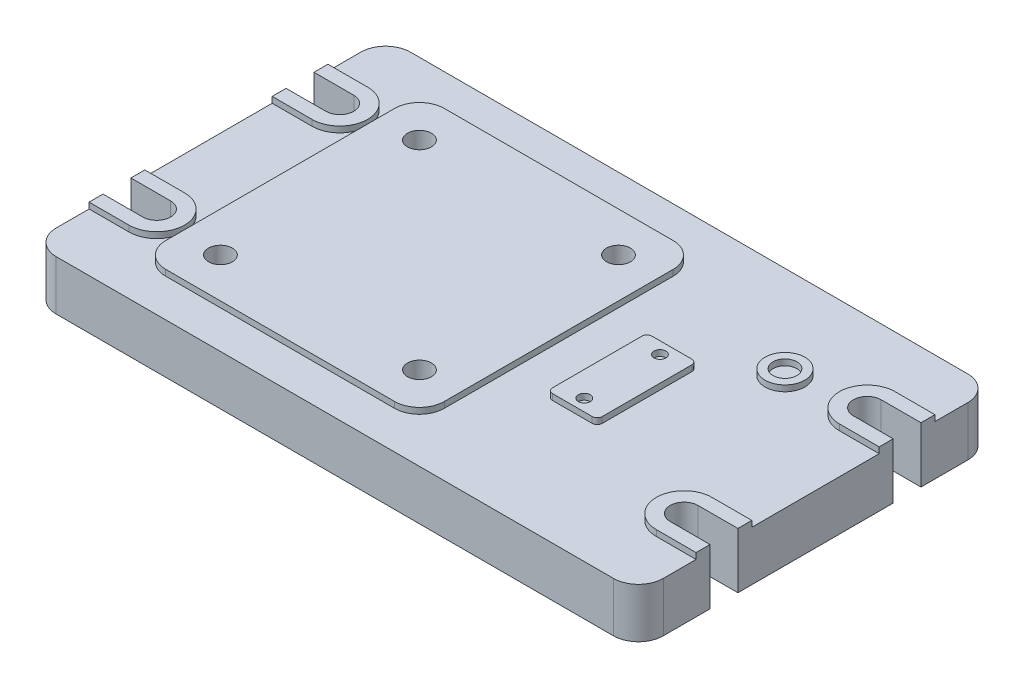
SolidWorks part; units mm, degrees
material "Plain Carbon Steel"
ref_plane "Front Plane" through (0, 0, 0) normal (0, 0, 1) x (1, 0, 0)
ref_plane "Top Plane" through (0, 0, 0) normal (0, 1, 0) x (1, 0, 0)
ref_plane "Right Plane" through (0, 0, 0) normal (1, 0, 0) x (0, 0, -1)
sketch "Base Plate Profile Sketch" plane through (0, 0, 0) normal (0, 1, 0) x (1, 0, 0)
  line L0 (0, 321.8341) -> (0, -345.455) construction
  line L1 (627.6398, 0) -> (-439.5166, 0) construction
  line L2 (-152.5, 46) -> (-132.5, 46) construction
  line L3 (-152.5, 89) -> (152.5, 89)
  line L4 (-152.5, 89) -> (-152.5, -89)
  line L5 (-152.5, -89) -> (152.5, -89)
  line L6 (152.5, 89) -> (152.5, -89)
  line L7 (-152.5, 89) -> (152.5, -89) construction
  line L8 (-152.5, -89) -> (152.5, 89) construction
  line L9 (-152.5, 53) -> (-132.5, 53)
  line L10 (-152.5, 39) -> (-132.5, 39)
  line L11 (-152.5, 53) -> (-152.5, 39)
  line L12 (152.5, 53) -> (132.5, 53)
  line L13 (152.5, 39) -> (132.5, 39)
  line L14 (152.5, 53) -> (152.5, 39)
  line L15 (152.5, -53) -> (152.5, -39)
  line L16 (152.5, -39) -> (132.5, -39)
  line L17 (152.5, -53) -> (132.5, -53)
  line L18 (-152.5, -53) -> (-132.5, -53)
  line L19 (-152.5, -39) -> (-132.5, -39)
  line L20 (-152.5, -53) -> (-152.5, -39)
  arc A1 (-132.5, 39) -> (-132.5, 53) centre (-132.5, 46) ccw
  arc A2 (132.5, 39) -> (132.5, 53) centre (132.5, 46) cw
  arc A3 (132.5, -39) -> (132.5, -53) centre (132.5, -46) ccw
  arc A4 (-132.5, -39) -> (-132.5, -53) centre (-132.5, -46) cw
  point P5 (0, 0)
  point P12 (-162.4479, 46)
  dimension "D5" = 7
  dimension "D1" = 178
  dimension "D2" = 305
  dimension "D3" = 20
  dimension "D4" = 43
  dimension "D6" = 314.9479
extrude "Base Plate 305x178x25" add sketch "Base Plate Profile Sketch" along normal blind 25 contours L19 A4 L18 L4 L5 L6 L17 A3 L16 L13 A2 L12 L3 L9 A1 L10
sketch "Round Boss Sketch" plane through (0, 25, 0) normal (0, 1, 0) x (1, 0, 0)
  line L0 (-152.5, 89) -> (-152.5, 53) construction
  line L1 (-152.5, 60) -> (-152.5, 53)
  line L2 (-152.5, 39) -> (-152.5, -39) construction
  line L3 (-152.5, 39) -> (-152.5, 32)
  line L4 (-152.5, 46) -> (-132.5, 46) construction
  line L5 (-152.5, 60) -> (-132.5, 60)
  line L6 (-152.5, 32) -> (-132.5, 32)
  line L7 (152.5, -53) -> (152.5, -89) construction
  line L8 (-152.5, -89) -> (152.5, -89) construction
  line L9 (-152.5, 53) -> (-132.5, 53) construction
  line L10 (-152.5, 53) -> (-132.5, 53)
  line L11 (-152.5, 39) -> (-132.5, 39) construction
  line L12 (-152.5, 39) -> (-132.5, 39)
  line L13 (0, 195.1549) -> (0, -170.1958) construction
  line L14 (185.9906, 0) -> (-179.3514, 0) construction
  line L15 (152.5, 53) -> (132.5, 53)
  line L16 (152.5, 60) -> (152.5, 53)
  line L17 (152.5, 60) -> (132.5, 60)
  line L18 (152.5, 32) -> (132.5, 32)
  line L19 (152.5, 39) -> (152.5, 32)
  line L20 (152.5, 39) -> (132.5, 39)
  line L21 (152.5, -39) -> (132.5, -39)
  line L22 (152.5, -39) -> (152.5, -32)
  line L23 (152.5, -32) -> (132.5, -32)
  line L24 (152.5, -60) -> (132.5, -60)
  line L25 (152.5, -60) -> (152.5, -53)
  line L26 (152.5, -53) -> (132.5, -53)
  line L27 (-152.5, -53) -> (-132.5, -53)
  line L28 (-152.5, -60) -> (-152.5, -53)
  line L29 (-152.5, -60) -> (-132.5, -60)
  line L30 (-152.5, -32) -> (-132.5, -32)
  line L31 (-152.5, -39) -> (-152.5, -32)
  line L32 (-152.5, -39) -> (-132.5, -39)
  line L33 (-152.5, -53) -> (-152.5, -89) construction
  line L34 (-152.5, -53) -> (-132.5, -53) construction
  arc A1 (-132.5, 32) -> (-132.5, 60) centre (-132.5, 46) ccw
  arc A2 (-132.5, 39) -> (-132.5, 53) centre (-132.5, 46) ccw construction
  arc A3 (-132.5, 39) -> (-132.5, 53) centre (-132.5, 46) ccw
  arc A4 (132.5, 39) -> (132.5, 53) centre (132.5, 46) cw
  arc A5 (132.5, 32) -> (132.5, 60) centre (132.5, 46) cw
  arc A6 (132.5, -32) -> (132.5, -60) centre (132.5, -46) ccw
  arc A7 (132.5, -39) -> (132.5, -53) centre (132.5, -46) ccw
  arc A8 (-132.5, -39) -> (-132.5, -53) centre (-132.5, -46) cw
  arc A9 (-132.5, -32) -> (-132.5, -60) centre (-132.5, -46) cw
  point P7 (-142.5, 46)
  dimension "D1" = 14
  dimension "D2" = 36
  dimension "D3" = 10
  dimension "D4" = 7
extrude "Round Boss 3mm" add sketch "Round Boss Sketch" along normal blind 3
sketch "Raised Pads Sketch" plane through (0, 25, 0) normal (0, 1, 0) x (1, 0, 0)
  line L0 (-152.5, -60) -> (-152.5, -89) construction
  line L1 (-104, 70) -> (11, 70)
  line L2 (-116.5, 57.5) -> (-116.5, -57.5)
  line L3 (-104, -70) -> (11, -70)
  line L4 (23.5, 57.5) -> (23.5, -57.5)
  line L5 (-116.5, 70) -> (23.5, -70) construction
  line L6 (-116.5, -70) -> (23.5, 70) construction
  line L7 (0, 0) -> (-206.4428, 0) construction
  line L8 (-46.5, 70) -> (-46.5, -52.4573) construction
  line L11 (40.3696, -1.9083) -> (77.4213, -1.9083) construction
  line L12 (47.2286, 23.0917) -> (67.2286, 23.0917)
  line L13 (44.7286, 20.5917) -> (44.7286, -24.4083)
  line L14 (47.2286, -26.9083) -> (67.2286, -26.9083)
  line L15 (69.7286, 20.5917) -> (69.7286, -24.4083)
  line L16 (44.7286, 23.0917) -> (69.7286, -26.9083) construction
  line L17 (44.7286, -26.9083) -> (69.7286, 23.0917) construction
  arc A0 (-116.5, -57.5) -> (-104, -70) centre (-104, -57.5) ccw
  arc A1 (11, -70) -> (23.5, -57.5) centre (11, -57.5) ccw
  arc A2 (23.5, 57.5) -> (11, 70) centre (11, 57.5) ccw
  arc A3 (-116.5, 57.5) -> (-104, 70) centre (-104, 57.5) cw
  circle A4 centre (-96.5, 50) radius 6
  circle A5 centre (-96.5, -50) radius 6
  circle A6 centre (3.5, -50) radius 6
  circle A7 centre (3.5, 50) radius 6
  circle A8 centre (57.2286, 17.0917) radius 3
  circle A9 centre (57.2286, -20.9083) radius 3
  arc A10 (67.2286, 23.0917) -> (69.7286, 20.5917) centre (67.2286, 20.5917) cw
  arc A11 (67.2286, -26.9083) -> (69.7286, -24.4083) centre (67.2286, -24.4083) ccw
  arc A12 (47.2286, -26.9083) -> (44.7286, -24.4083) centre (47.2286, -24.4083) cw
  arc A13 (47.2286, 23.0917) -> (44.7286, 20.5917) centre (47.2286, 20.5917) ccw
  circle A14 centre (94.8095, 42.3424) radius 10
  circle A15 centre (94.8095, 42.3424) radius 6
  point P0 (-46.5, 0)
  point P5 (-46.5, -70)
  point P33 (57.2286, -1.9083)
  dimension "D4" = 12.5
  dimension "D7" = 12
  dimension "D8" = 12
  dimension "D11" = 6
  dimension "D12" = 6
  dimension "D13" = 38
  dimension "D14" = 2.5
  dimension "D15" = 20
  dimension "D16" = 12
  dimension "D1" = 106
  dimension "D2" = 140
  dimension "D3" = 140
  dimension "D5" = 100
  dimension "D6" = 50
  dimension "D9" = 25
  dimension "D10" = 50
  dimension "D17" = 206.4428
  dimension "D18" = 52.4573
  dimension "D19" = 57.2286
  dimension "D20" = 1.9083
  dimension "D21" = 37.0517
  dimension "D22" = 16.859
  dimension "D23" = 94.8095
  dimension "D24" = 42.3424
extrude "Raised Pads 3mm" add sketch "Raised Pads Sketch" along normal blind 3
fillet "Corner Fillets R12.5" radius 12.5 4 edges at (-152.5, 12.5, -89) (152.5, 12.5, -89) (152.5, 12.5, 89) (-152.5, 12.5, 89)
sketch "Slot Recess Sketch" plane through (0, 0, 0) normal (0, -1, 0) x (1, 0, 0)
  line L0 (-133.5, 25) -> (-133.5, -25)
  line L1 (-133.5, -25) -> (-116.5, -25)
  line L2 (-116.5, -25) -> (-116.5, -70)
  line L3 (-116.5, -70) -> (116.5, -70)
  line L4 (-133.5, 25) -> (-116.5, 25)
  line L5 (-116.5, 25) -> (-116.5, 70)
  line L6 (-116.5, 70) -> (116.5, 70)
  line L7 (0, 0) -> (-183.8119, 0) construction
  line L8 (-152.5, -39) -> (-152.5, 39) construction
  line L9 (-152.5, -76.5) -> (-152.5, -53) construction
  line L10 (-152.5, 53) -> (-152.5, 76.5) construction
  line L11 (0, 105.3287) -> (0, -118.2776) construction
  line L12 (116.5, -25) -> (116.5, -70)
  line L13 (133.5, -25) -> (116.5, -25)
  line L14 (133.5, 25) -> (133.5, -25)
  line L15 (133.5, 25) -> (116.5, 25)
  line L16 (116.5, 25) -> (116.5, 70)
  point P21 (0, -70)
  point P25 (0, 70)
  dimension "D1" = 50
  dimension "D2" = 19
  dimension "D3" = 36
  dimension "D4" = 36
  dimension "D5" = 140
extrude "Slot Recesses 10 Deep" cut sketch "Slot Recess Sketch" against normal blind 10
sketch "Pad Hole A Position Sketch" plane through (0, 25, 0) normal (0, 1, 0) x (1, 0, 0)
  circle A0 centre (-96.5, -50) radius 7
  dimension "D1" = 14
extrude "Pad Hole A" cut sketch "Pad Hole A Position Sketch" along normal blind 10 from offset 18 contours A0 offset against normal yes
sketch "Pad Hole B Position Sketch" plane through (0, 25, 0) normal (0, 1, 0) x (1, 0, 0)
  circle A0 centre (-96.5, -50) radius 6 construction
  circle A1 centre (-96.5, -50) radius 6
extrude "Pad Hole B" cut sketch "Pad Hole B Position Sketch" against normal up to next
ref_plane "Plane2" through (-46.5, 0, 0) normal (-1, 0, 0) x (0, 0, 1)
mirror "Pad Holes Mirror 1" about plane through (-46.5, 0, 0) normal (-1, 0, 0) of "Pad Hole A", "Pad Hole B"
ref_plane "Plane3" through (0, 0, 0) normal (0, 0, 1) x (1, 0, 0)
mirror "Pad Holes Mirror 2" about plane through (0, 0, 0) normal (0, 0, 1) of "Pad Holes Mirror 1", "Pad Hole B", "Pad Hole A"
